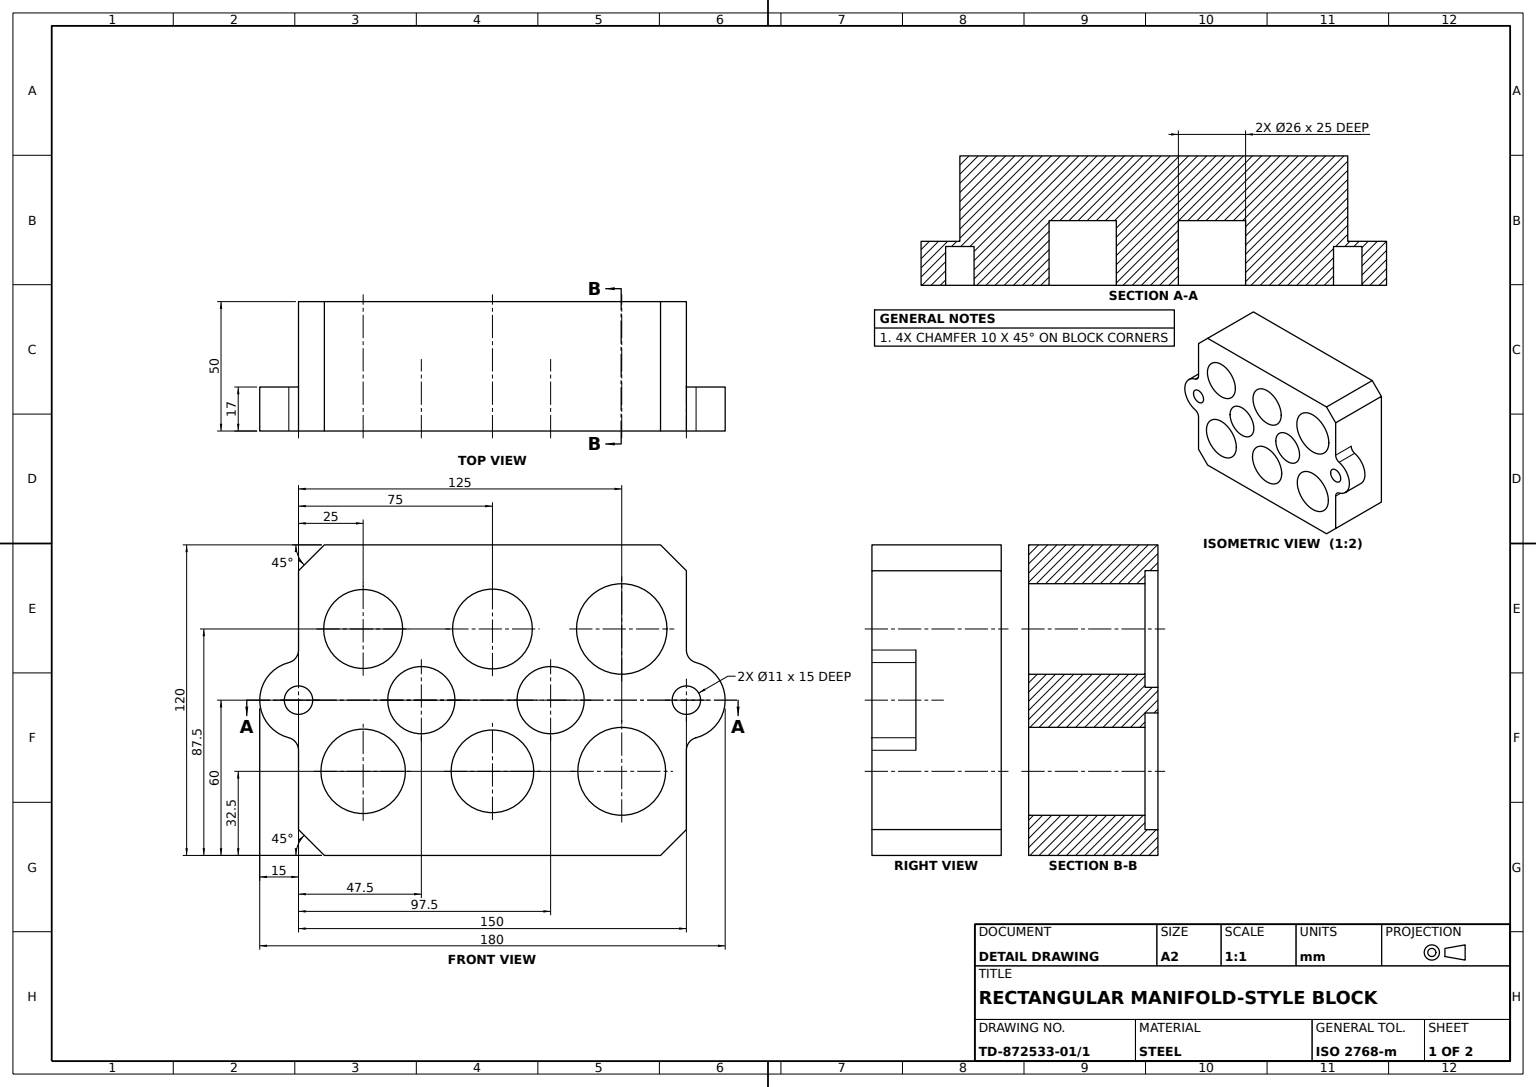
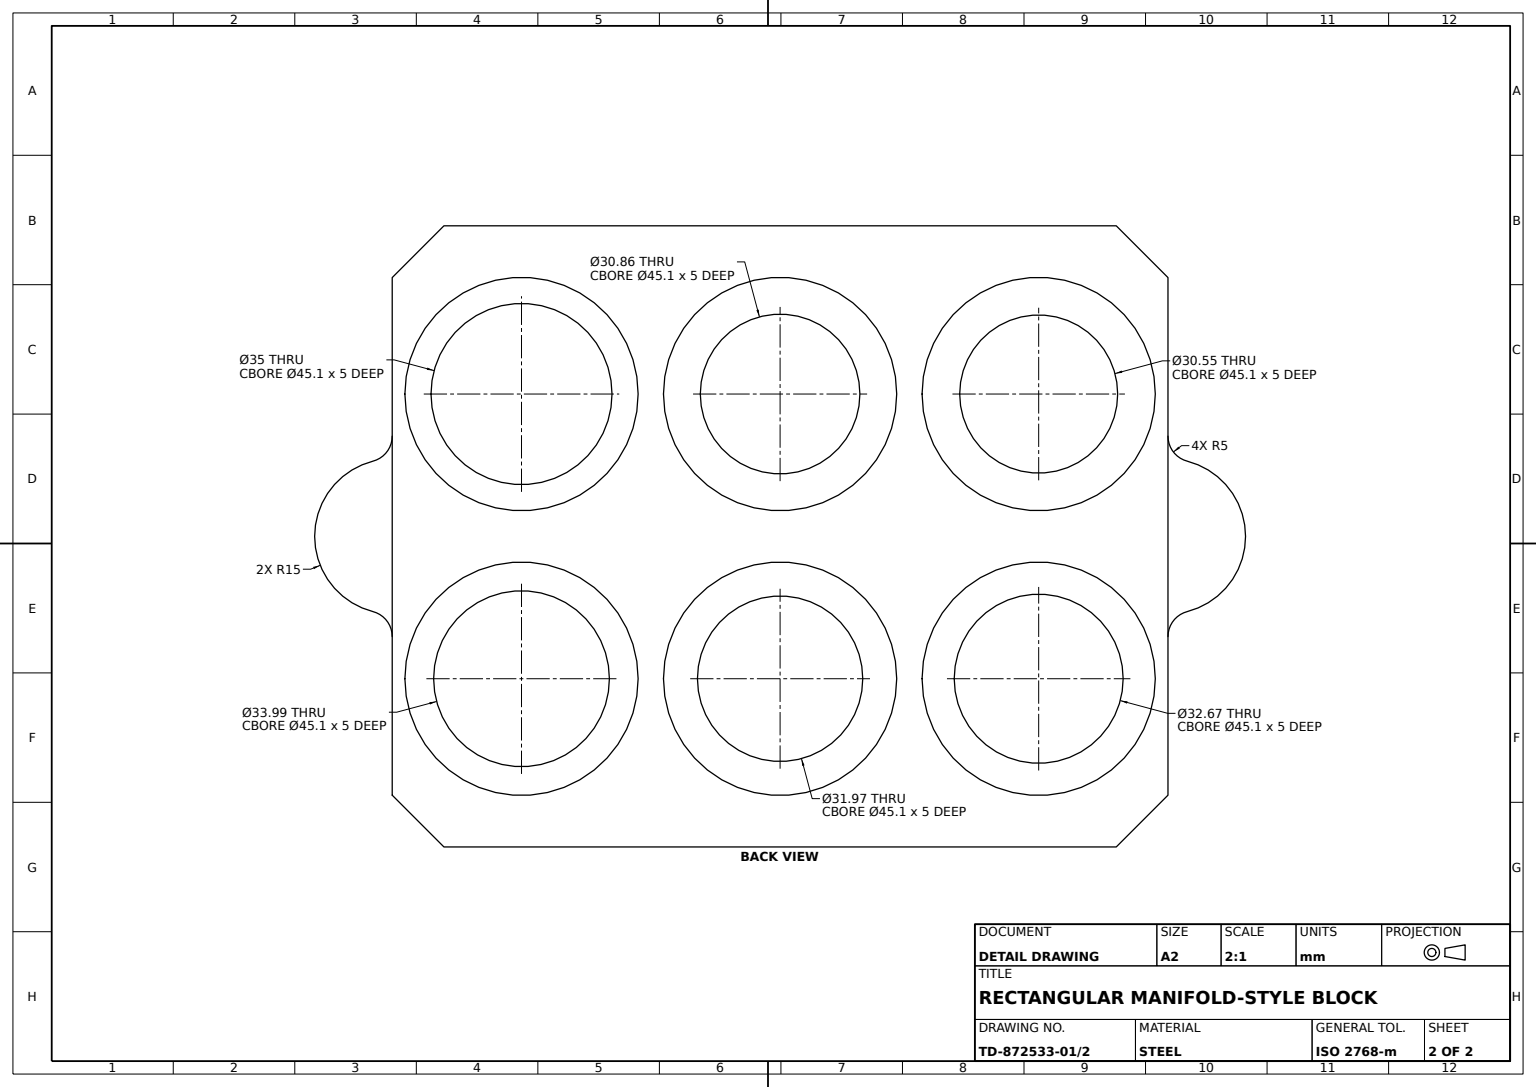
SolidWorks part; units mm, degrees
material "Plain Carbon Steel"
ref_plane "Front Plane" through (0, 0, 0) normal (0, 0, 1) x (1, 0, 0)
ref_plane "Top Plane" through (0, 0, 0) normal (0, 1, 0) x (1, 0, 0)
ref_plane "Right Plane" through (0, 0, 0) normal (1, 0, 0) x (0, 0, -1)
sketch "Block Profile Sketch" plane through (0, 0, 0) normal (0, 0, 1) x (1, 0, 0)
  line L1 (0, 0) -> (150, 0)
  line L2 (0, 0) -> (0, 120)
  line L3 (0, 120) -> (150, 120)
  line L4 (150, 0) -> (150, 120)
  dimension "D1" = 150
  dimension "D2" = 120
extrude "Base Block 150x120x50" add sketch "Block Profile Sketch" along normal blind 50
sketch "Port Counterbore Sketch" plane through (0, 0, 0) normal (0, 0, -1) x (-1, 0, 0)
  line L2 (-125, 124.3797) -> (-125, -7.917) construction
  line L3 (-75, 127.2378) -> (-75, -13.6051) construction
  line L4 (-25, 130.5488) -> (-25, -13.6051) construction
  line L5 (-165.4145, 87.5) -> (22.8005, 87.5) construction
  line L6 (-162.6129, 60) -> (22.8005, 60) construction
  line L7 (-159.0473, 32.5) -> (16.688, 32.5) construction
  line L8 (0, 0) -> (-150, 0) construction
  line L9 (-150, 0) -> (-150, 120) construction
  circle A9 centre (-125, 87.5) radius 22.55
  circle A10 centre (-75, 87.5) radius 22.55
  circle A11 centre (-25, 87.5) radius 22.55
  circle A12 centre (-25, 32.5) radius 22.55
  circle A13 centre (-75, 32.5) radius 22.55
  circle A14 centre (-125, 32.5) radius 22.55
  dimension "D8" = 45.1
  dimension "D1" = 32.5
  dimension "D2" = 60
  dimension "D3" = 87.5
  dimension "D4" = 25
  dimension "D5" = 75
  dimension "D6" = 125
extrude "Port Counterbores 5 Deep" cut sketch "Port Counterbore Sketch" against normal blind 5
sketch "Port Hole Sketch" plane through (0, 0, 5) normal (0, 0, -1) x (-1, 0, 0)
  circle A0 centre (-125, 87.5) radius 17.5
  circle A1 centre (-75, 87.5) radius 15.429
  circle A2 centre (-25, 87.5) radius 15.2743
  circle A3 centre (-125, 32.5) radius 16.9931
  circle A4 centre (-75, 32.5) radius 15.9826
  circle A5 centre (-25, 32.5) radius 16.3336
  circle A6 centre (-125, 87.5) radius 22.55 construction
  circle A7 centre (-75, 87.5) radius 22.55 construction
  circle A8 centre (-25, 87.5) radius 22.55 construction
  circle A9 centre (-125, 32.5) radius 22.55 construction
  circle A10 centre (-75, 32.5) radius 22.55 construction
  circle A11 centre (-25, 32.5) radius 22.55 construction
  dimension "D1" = 35
  dimension "D2" = 33.9862
  dimension "D3" = 32.6672
  dimension "D4" = 31.9653
  dimension "D5" = 30.858
  dimension "D6" = 30.5485
extrude "Port Through Holes" cut sketch "Port Hole Sketch" against normal through all
chamfer "Edge Chamfer 10x45 A" distance 10 angle 45 1 edges at (0, 0, 25)
chamfer "Edge Chamfer 10x45 B" distance 10 angle 45 3 edges at (0, 120, 25) (150, 120, 25) (150, 0, 25)
sketch "Mounting Ear Profile Sketch" plane through (0, 0, 50) normal (0, 0, 1) x (1, 0, 0)
  line L0 (0, 110) -> (0, 10) construction
  line L1 (0, 79.3649) -> (0, 40.6351)
  line L2 (75, 120) -> (75, 0) construction
  line L3 (140, 120) -> (10, 120) construction
  line L4 (10, 0) -> (140, 0) construction
  line L5 (150, 79.3649) -> (150, 40.6351)
  arc A0 (-3.75, 74.5237) -> (-3.75, 45.4763) centre (0, 60) ccw
  arc A1 (-3.75, 45.4763) -> (0, 40.6351) centre (-5, 40.6351) cw
  arc A2 (-3.75, 74.5237) -> (0, 79.3649) centre (-5, 79.3649) ccw
  arc A3 (153.75, 74.5237) -> (150, 79.3649) centre (155, 79.3649) cw
  arc A4 (153.75, 74.5237) -> (153.75, 45.4763) centre (150, 60) cw
  arc A5 (153.75, 45.4763) -> (150, 40.6351) centre (155, 40.6351) ccw
  point P6 (0, 60)
  dimension "D1" = 15
  dimension "D2" = 5
  dimension "D3" = 5
extrude "Mounting Ears" add sketch "Mounting Ear Profile Sketch" against normal blind 17
sketch "Ear Hole Sketch" plane through (0, 0, 50) normal (0, 0, 1) x (1, 0, 0)
  circle A0 centre (150, 60) radius 5.5
  circle A1 centre (0, 60) radius 5.5
  arc A2 (-3.75, 74.5237) -> (-3.75, 45.4763) centre (0, 60) ccw construction
  arc A3 (153.75, 45.4763) -> (153.75, 74.5237) centre (150, 60) ccw construction
  dimension "D1" = 11
extrude "Ear Holes" cut sketch "Ear Hole Sketch" against normal blind 15
sketch "Side Recess Sketch" plane through (0, 0, 50) normal (0, 0, 1) x (1, 0, 0)
  line L0 (0, 60) -> (150, 60) construction
  circle A1 centre (47.5, 60) radius 13
  circle A2 centre (97.5, 60) radius 13
  dimension "D1" = 26
  dimension "D2" = 102.5
  dimension "D3" = 52.5
extrude "Side Recess" cut sketch "Side Recess Sketch" against normal blind 25
